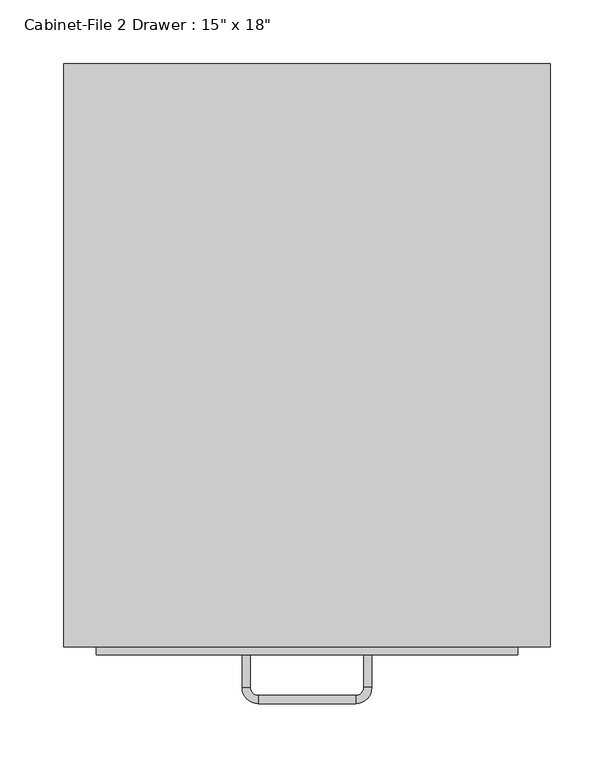
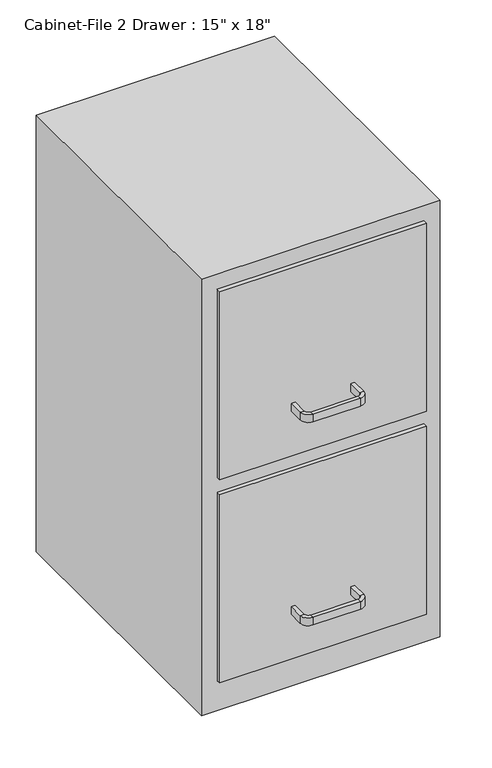
"""IFC4 building model written with IfcOpenShell, lengths in millimetres: furniture geometry."""

from ifc_helpers import new_model, si_unit, frame, origin, origin_with_axes, place, context, project, spatial, polyline, circle_curve, outline, extrude, source, transform, mapped, element, save
from ifc_brep_helpers import plane_surface, cylinder_surface, revolved_surface, advanced_brep


def furniture_bb55ed6b(model_context):
    return source(origin(), model_context, "Body", "SolidModel", [
        extrude(outline(polyline([(37.203553, -377.0843001), (-292.996447, -377.0843001), (-292.996447, -370.7343001), (37.203553, -370.7343001), (37.203553, -377.0843001)])), frame((0.0, 0.0, 393.7), z_axis=(0.0, 0.0, 1.0), x_axis=(1.0, 0.0, 0.0)), (0.0, 0.0, 1.0), 317.5),
        extrude(outline(polyline([(37.203553, -377.0843001), (-292.996447, -377.0843001), (-292.996447, -370.7343001), (37.203553, -370.7343001), (37.203553, -377.0843001)])), frame((0.0, 0.0, 50.8), z_axis=(0.0, 0.0, 1.0), x_axis=(1.0, 0.0, 0.0)), (0.0, 0.0, 1.0), 317.5),
        advanced_brep(
        [(-172.346447, -377.0843001, 127.0), (-178.696447, -377.0843001, 127.0), (-178.696447, -377.0843001, 139.7), (-172.346447, -377.0843001, 139.7), (-172.346447, -402.4843001, 127.0), (-178.696447, -402.4843001, 127.0), (-178.696447, -402.4843001, 139.7), (-172.346447, -402.4843001, 139.7), (-165.996447, -415.1843001, 127.0), (-165.996447, -408.8343001, 127.0), (-165.996447, -415.1843001, 139.7), (-165.996447, -408.8343001, 139.7), (-89.796447, -408.8343001, 127.0), (-89.796447, -415.1843001, 127.0), (-89.796447, -415.1843001, 139.7), (-89.796447, -408.8343001, 139.7), (-77.096447, -402.4843001, 127.0), (-83.446447, -402.4843001, 127.0), (-77.096447, -402.4843001, 139.7), (-83.446447, -402.4843001, 139.7), (-83.446447, -377.0843001, 127.0), (-83.446447, -377.0843001, 139.7), (-77.096447, -377.0843001, 139.7), (-77.096447, -377.0843001, 127.0)],
        [
            (0, 1),
            (1, 2),
            (2, 3),
            (3, 0),
            (0, 4),
            (4, 5),
            (5, 1),
            (5, 6),
            (6, 2),
            (6, 7),
            (7, 3),
            (7, 4),
            (8, 5, circle_curve(frame((-165.996447, -402.4843001, 127.0), z_axis=(0.0, 0.0, -1.0), x_axis=(-1.0, 0.0, 0.0)), 12.7)),
            (4, 9, circle_curve(frame((-165.996447, -402.4843001, 127.0), z_axis=(0.0, 0.0, 1.0), x_axis=(-1.0, 0.0, 0.0)), 6.35)),
            (9, 8),
            (10, 6, circle_curve(frame((-165.996447, -402.4843001, 139.7), z_axis=(0.0, 0.0, -1.0), x_axis=(-1.0, 0.0, 0.0)), 12.7)),
            (8, 10),
            (11, 7, circle_curve(frame((-165.996447, -402.4843001, 139.7), z_axis=(0.0, 0.0, -1.0), x_axis=(-1.0, 0.0, 0.0)), 6.35)),
            (10, 11),
            (11, 9),
            (9, 12),
            (12, 13),
            (13, 8),
            (13, 14),
            (14, 10),
            (14, 15),
            (15, 11),
            (15, 12),
            (16, 13, circle_curve(frame((-89.796447, -402.4843001, 127.0), z_axis=(0.0, 0.0, -1.0), x_axis=(0.0, -1.0, 0.0)), 12.7)),
            (12, 17, circle_curve(frame((-89.796447, -402.4843001, 127.0), z_axis=(0.0, 0.0, 1.0), x_axis=(0.0, -1.0, 0.0)), 6.35)),
            (17, 16),
            (18, 14, circle_curve(frame((-89.796447, -402.4843001, 139.7), z_axis=(0.0, 0.0, -1.0), x_axis=(0.0, -1.0, 0.0)), 12.7)),
            (16, 18),
            (19, 15, circle_curve(frame((-89.796447, -402.4843001, 139.7), z_axis=(0.0, 0.0, -1.0), x_axis=(0.0, -1.0, 0.0)), 6.35)),
            (18, 19),
            (19, 17),
            (20, 21),
            (21, 22),
            (22, 23),
            (23, 20),
            (17, 20),
            (23, 16),
            (22, 18),
            (21, 19),
        ],
        [
            plane_surface(frame((-661.3382215, -377.0843001, 0.0), z_axis=(0.0, 1.0, 0.0), x_axis=(0.0, 0.0, -1.0))),
            plane_surface(frame((-172.346447, -377.0843001, 127.0), z_axis=(0.0, 0.0, -1.0), x_axis=(0.0, -1.0, 0.0))),
            plane_surface(frame((-178.696447, -377.0843001, 127.0), z_axis=(-1.0, 0.0, 0.0), x_axis=(0.0, -1.0, 0.0))),
            plane_surface(frame((-178.696447, -377.0843001, 139.7), z_axis=(0.0, 0.0, 1.0), x_axis=(0.0, -1.0, 0.0))),
            plane_surface(frame((-172.346447, -377.0843001, 139.7), z_axis=(1.0, 0.0, 0.0), x_axis=(0.0, -1.0, 0.0))),
            plane_surface(frame((-165.996447, -402.4843001, 127.0), z_axis=(0.0, 0.0, -1.0), x_axis=(-1.0, 0.0, 0.0))),
            cylinder_surface(frame((-165.996447, -402.4843001, 0.0), z_axis=(0.0, 0.0, 1.0), x_axis=(-1.0, 0.0, 0.0)), 12.7),
            plane_surface(frame((-165.996447, -402.4843001, 139.7), z_axis=(0.0, 0.0, 1.0), x_axis=(-1.0, 0.0, 0.0))),
            revolved_surface(polyline([(-172.34644699999998, -402.4843001, 139.7), (-172.34644699999998, -402.4843001, 127.0)]), (-165.996447, -402.4843001, 0.0), (0.0, 0.0, 1.0)),
            plane_surface(frame((-165.996447, -408.8343001, 127.0), z_axis=(0.0, 0.0, -1.0), x_axis=(1.0, 0.0, 0.0))),
            plane_surface(frame((-165.996447, -415.1843001, 127.0), z_axis=(0.0, -1.0, 0.0), x_axis=(1.0, 0.0, 0.0))),
            plane_surface(frame((-165.996447, -415.1843001, 139.7), z_axis=(0.0, 0.0, 1.0), x_axis=(1.0, 0.0, 0.0))),
            plane_surface(frame((-165.996447, -408.8343001, 139.7), z_axis=(0.0, 1.0, 0.0), x_axis=(1.0, 0.0, 0.0))),
            plane_surface(frame((-89.796447, -402.4843001, 127.0), z_axis=(0.0, 0.0, -1.0), x_axis=(0.0, -1.0, 0.0))),
            cylinder_surface(frame((-89.796447, -402.4843001, 0.0), z_axis=(0.0, 0.0, 1.0), x_axis=(0.0, -1.0, 0.0)), 12.7),
            plane_surface(frame((-89.796447, -402.4843001, 139.7), z_axis=(0.0, 0.0, 1.0), x_axis=(0.0, -1.0, 0.0))),
            revolved_surface(polyline([(-89.796447, -408.8343001, 139.7), (-89.796447, -408.8343001, 127.0)]), (-89.796447, -402.4843001, 0.0), (0.0, 0.0, 1.0)),
            plane_surface(frame((-559.7382215, -377.0843001, 0.0), z_axis=(0.0, 1.0, 0.0), x_axis=(0.0, 0.0, 1.0))),
            plane_surface(frame((-83.446447, -402.4843001, 127.0), z_axis=(0.0, 0.0, -1.0), x_axis=(0.0, 1.0, 0.0))),
            plane_surface(frame((-77.096447, -402.4843001, 127.0), z_axis=(1.0, 0.0, 0.0), x_axis=(0.0, 1.0, 0.0))),
            plane_surface(frame((-77.096447, -402.4843001, 139.7), z_axis=(0.0, 0.0, 1.0), x_axis=(0.0, 1.0, 0.0))),
            plane_surface(frame((-83.446447, -402.4843001, 139.7), z_axis=(-1.0, 0.0, 0.0), x_axis=(0.0, 1.0, 0.0))),
        ],
        [
            (0, [[1, 2, 3, 4]]),
            (1, [[-1, 5, 6, 7]]),
            (2, [[-2, -7, 8, 9]]),
            (3, [[-3, -9, 10, 11]]),
            (4, [[-4, -11, 12, -5]]),
            (5, [[13, -6, 14, 15]]),
            (6, [[16, -8, -13, 17]]),
            (7, [[18, -10, -16, 19]]),
            (8, [[-14, -12, -18, 20]]),
            (9, [[-15, 21, 22, 23]]),
            (10, [[-17, -23, 24, 25]]),
            (11, [[-19, -25, 26, 27]]),
            (12, [[-20, -27, 28, -21]]),
            (13, [[29, -22, 30, 31]]),
            (14, [[32, -24, -29, 33]]),
            (15, [[34, -26, -32, 35]]),
            (16, [[-30, -28, -34, 36]]),
            (17, [[37, 38, 39, 40]]),
            (18, [[-31, 41, -40, 42]]),
            (19, [[-33, -42, -39, 43]]),
            (20, [[-35, -43, -38, 44]]),
            (21, [[-36, -44, -37, -41]]),
        ],
    ),
        advanced_brep(
        [(-172.346447, -377.0843001, 469.9), (-178.696447, -377.0843001, 469.9), (-178.696447, -377.0843001, 482.6), (-172.346447, -377.0843001, 482.6), (-172.346447, -402.4843001, 469.9), (-178.696447, -402.4843001, 469.9), (-178.696447, -402.4843001, 482.6), (-172.346447, -402.4843001, 482.6), (-165.996447, -415.1843001, 469.9), (-165.996447, -408.8343001, 469.9), (-165.996447, -415.1843001, 482.6), (-165.996447, -408.8343001, 482.6), (-89.796447, -408.8343001, 469.9), (-89.796447, -415.1843001, 469.9), (-89.796447, -415.1843001, 482.6), (-89.796447, -408.8343001, 482.6), (-77.096447, -402.4843001, 469.9), (-83.446447, -402.4843001, 469.9), (-77.096447, -402.4843001, 482.6), (-83.446447, -402.4843001, 482.6), (-83.446447, -377.0843001, 469.9), (-83.446447, -377.0843001, 482.6), (-77.096447, -377.0843001, 482.6), (-77.096447, -377.0843001, 469.9)],
        [
            (0, 1),
            (1, 2),
            (2, 3),
            (3, 0),
            (0, 4),
            (4, 5),
            (5, 1),
            (5, 6),
            (6, 2),
            (6, 7),
            (7, 3),
            (7, 4),
            (8, 5, circle_curve(frame((-165.996447, -402.4843001, 469.9), z_axis=(0.0, 0.0, -1.0), x_axis=(-1.0, 0.0, 0.0)), 12.7)),
            (4, 9, circle_curve(frame((-165.996447, -402.4843001, 469.9), z_axis=(0.0, 0.0, 1.0), x_axis=(-1.0, 0.0, 0.0)), 6.35)),
            (9, 8),
            (10, 6, circle_curve(frame((-165.996447, -402.4843001, 482.6), z_axis=(0.0, 0.0, -1.0), x_axis=(-1.0, 0.0, 0.0)), 12.7)),
            (8, 10),
            (11, 7, circle_curve(frame((-165.996447, -402.4843001, 482.6), z_axis=(0.0, 0.0, -1.0), x_axis=(-1.0, 0.0, 0.0)), 6.35)),
            (10, 11),
            (11, 9),
            (9, 12),
            (12, 13),
            (13, 8),
            (13, 14),
            (14, 10),
            (14, 15),
            (15, 11),
            (15, 12),
            (16, 13, circle_curve(frame((-89.796447, -402.4843001, 469.9), z_axis=(0.0, 0.0, -1.0), x_axis=(0.0, -1.0, 0.0)), 12.7)),
            (12, 17, circle_curve(frame((-89.796447, -402.4843001, 469.9), z_axis=(0.0, 0.0, 1.0), x_axis=(0.0, -1.0, 0.0)), 6.35)),
            (17, 16),
            (18, 14, circle_curve(frame((-89.796447, -402.4843001, 482.6), z_axis=(0.0, 0.0, -1.0), x_axis=(0.0, -1.0, 0.0)), 12.7)),
            (16, 18),
            (19, 15, circle_curve(frame((-89.796447, -402.4843001, 482.6), z_axis=(0.0, 0.0, -1.0), x_axis=(0.0, -1.0, 0.0)), 6.35)),
            (18, 19),
            (19, 17),
            (20, 21),
            (21, 22),
            (22, 23),
            (23, 20),
            (17, 20),
            (23, 16),
            (22, 18),
            (21, 19),
        ],
        [
            plane_surface(frame((-661.3382215, -377.0843001, 0.0), z_axis=(0.0, 1.0, 0.0), x_axis=(0.0, 0.0, -1.0))),
            plane_surface(frame((-172.346447, -377.0843001, 469.9), z_axis=(0.0, 0.0, -1.0), x_axis=(0.0, -1.0, 0.0))),
            plane_surface(frame((-178.696447, -377.0843001, 469.9), z_axis=(-1.0, 0.0, 0.0), x_axis=(0.0, -1.0, 0.0))),
            plane_surface(frame((-178.696447, -377.0843001, 482.6), z_axis=(0.0, 0.0, 1.0), x_axis=(0.0, -1.0, 0.0))),
            plane_surface(frame((-172.346447, -377.0843001, 482.6), z_axis=(1.0, 0.0, 0.0), x_axis=(0.0, -1.0, 0.0))),
            plane_surface(frame((-165.996447, -402.4843001, 469.9), z_axis=(0.0, 0.0, -1.0), x_axis=(-1.0, 0.0, 0.0))),
            cylinder_surface(frame((-165.996447, -402.4843001, 0.0), z_axis=(0.0, 0.0, 1.0), x_axis=(-1.0, 0.0, 0.0)), 12.7),
            plane_surface(frame((-165.996447, -402.4843001, 482.6), z_axis=(0.0, 0.0, 1.0), x_axis=(-1.0, 0.0, 0.0))),
            revolved_surface(polyline([(-172.34644699999998, -402.4843001, 482.6), (-172.34644699999998, -402.4843001, 469.9)]), (-165.996447, -402.4843001, 0.0), (0.0, 0.0, 1.0)),
            plane_surface(frame((-165.996447, -408.8343001, 469.9), z_axis=(0.0, 0.0, -1.0), x_axis=(1.0, 0.0, 0.0))),
            plane_surface(frame((-165.996447, -415.1843001, 469.9), z_axis=(0.0, -1.0, 0.0), x_axis=(1.0, 0.0, 0.0))),
            plane_surface(frame((-165.996447, -415.1843001, 482.6), z_axis=(0.0, 0.0, 1.0), x_axis=(1.0, 0.0, 0.0))),
            plane_surface(frame((-165.996447, -408.8343001, 482.6), z_axis=(0.0, 1.0, 0.0), x_axis=(1.0, 0.0, 0.0))),
            plane_surface(frame((-89.796447, -402.4843001, 469.9), z_axis=(0.0, 0.0, -1.0), x_axis=(0.0, -1.0, 0.0))),
            cylinder_surface(frame((-89.796447, -402.4843001, 0.0), z_axis=(0.0, 0.0, 1.0), x_axis=(0.0, -1.0, 0.0)), 12.7),
            plane_surface(frame((-89.796447, -402.4843001, 482.6), z_axis=(0.0, 0.0, 1.0), x_axis=(0.0, -1.0, 0.0))),
            revolved_surface(polyline([(-89.796447, -408.8343001, 482.6), (-89.796447, -408.8343001, 469.9)]), (-89.796447, -402.4843001, 0.0), (0.0, 0.0, 1.0)),
            plane_surface(frame((-559.7382215, -377.0843001, 0.0), z_axis=(0.0, 1.0, 0.0), x_axis=(0.0, 0.0, 1.0))),
            plane_surface(frame((-83.446447, -402.4843001, 469.9), z_axis=(0.0, 0.0, -1.0), x_axis=(0.0, 1.0, 0.0))),
            plane_surface(frame((-77.096447, -402.4843001, 469.9), z_axis=(1.0, 0.0, 0.0), x_axis=(0.0, 1.0, 0.0))),
            plane_surface(frame((-77.096447, -402.4843001, 482.6), z_axis=(0.0, 0.0, 1.0), x_axis=(0.0, 1.0, 0.0))),
            plane_surface(frame((-83.446447, -402.4843001, 482.6), z_axis=(-1.0, 0.0, 0.0), x_axis=(0.0, 1.0, 0.0))),
        ],
        [
            (0, [[1, 2, 3, 4]]),
            (1, [[-1, 5, 6, 7]]),
            (2, [[-2, -7, 8, 9]]),
            (3, [[-3, -9, 10, 11]]),
            (4, [[-4, -11, 12, -5]]),
            (5, [[13, -6, 14, 15]]),
            (6, [[16, -8, -13, 17]]),
            (7, [[18, -10, -16, 19]]),
            (8, [[-14, -12, -18, 20]]),
            (9, [[-15, 21, 22, 23]]),
            (10, [[-17, -23, 24, 25]]),
            (11, [[-19, -25, 26, 27]]),
            (12, [[-20, -27, 28, -21]]),
            (13, [[29, -22, 30, 31]]),
            (14, [[32, -24, -29, 33]]),
            (15, [[34, -26, -32, 35]]),
            (16, [[-30, -28, -34, 36]]),
            (17, [[37, 38, 39, 40]]),
            (18, [[-31, 41, -40, 42]]),
            (19, [[-33, -42, -39, 43]]),
            (20, [[-35, -43, -38, 44]]),
            (21, [[-36, -44, -37, -41]]),
        ],
    ),
        extrude(outline(polyline([(62.603553, 86.4656999), (62.603553, -370.7343001), (-318.396447, -370.7343001), (-318.396447, 86.4656999), (62.603553, 86.4656999)])), origin_with_axes(), (0.0, 0.0, 1.0), 736.6),
    ])


if __name__ == "__main__":
    model = new_model("IFC4")
    model_context = context("Model", 3, world=origin())
    ifc_project = project(units=[si_unit("LENGTHUNIT", "METRE", prefix="MILLI")], contexts=[model_context])
    site = spatial("IfcSite", under=ifc_project)
    building = spatial("IfcBuilding", under=site)
    placement = place(None, origin())
    furniture_shape = furniture_bb55ed6b(model_context)
    element("IfcFurniture", 1, ObjectType="Cabinet-File 2 Drawer : 15\" x 18\"", at=placement, inside=building, context=model_context, shape_type="MappedRepresentation", body=[
        mapped(furniture_shape, transform((0.0, 0.0, 0.0), x_axis=(1.0, 0.0, 0.0), y_axis=(0.0, 1.0, 0.0), z_axis=(0.0, 0.0, 1.0))),
    ])
    save(model, "model.ifc")

# Revit data of these elements
# Type "Cabinet-File 2 Drawer : 15\" x 18\""
#   Assembly Code = "E2020200"
#   Depth = 1' - 6"
#   Height = 2' - 5"
#   Width = 1' - 3"
#   Cabinet Material = Steel, Paint Finish, Ivory, Glossy
#   Handle Material = Steel, Chrome Plated
#   Default Elevation = 0
# Element 1 (IfcFurniture, "Cabinet-File 2 Drawer : 15\" x 18\"")
#   Materials on its faces: "Steel, Chrome Plated", "Steel, Paint Finish, Ivory, Glossy"
# Materials
#   "Steel, Paint Finish, Ivory, Glossy": class "Metal", colour RGB 247 247 239, transparency 0, Description = "Steel, paint finish, ivory, glossy", Cost = 0
#   "Steel, Chrome Plated": class "Metal", colour RGB 17 17 17, transparency 0, Description = "Chromiuim plated steel", Cost = 0
